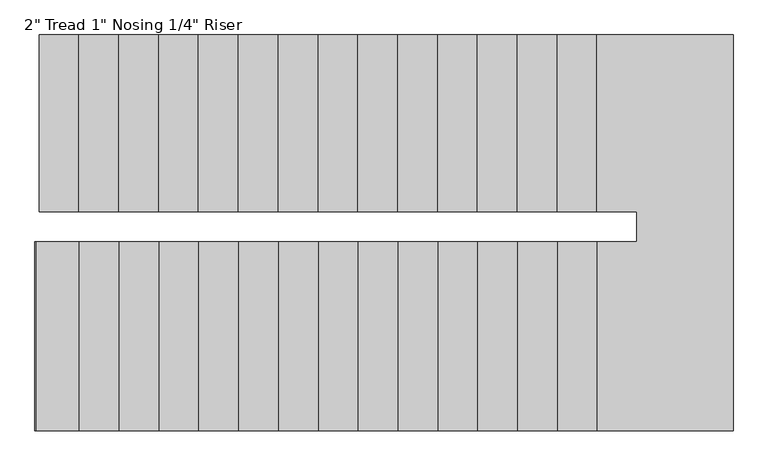
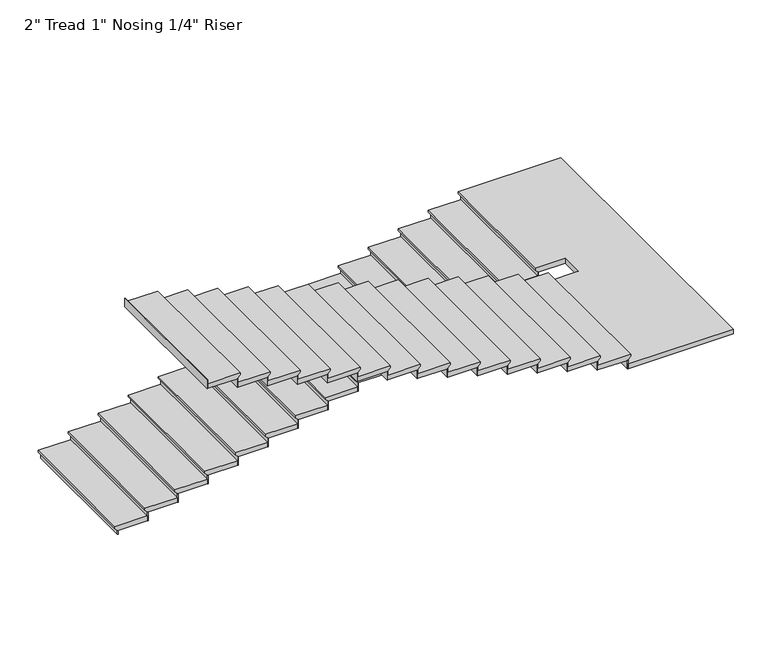
"""IFC4 building model written with IfcOpenShell, lengths in millimetres: stair flight geometry."""

from ifc_helpers import new_model, si_unit, origin, place, context, project, spatial, faceted_brep, source, transform, mapped, element, save


def stair_flight_8f1750f9(model_context):
    return source(origin(), model_context, "Body", "Brep", [
        faceted_brep([(-5254.0891351, 11154.2082924, 18360.39), (-5254.0891351, 11154.2082924, 18379.44), (-5254.0891351, 12506.0715905, 18379.44), (-5254.0891351, 12506.0715905, 18360.39), (-5228.6891351, 11154.2082924, 18334.99), (-5228.6891351, 12506.0715905, 18334.99), (-4923.8891351, 11154.2082924, 18379.44), (-4923.8891351, 12506.0715905, 18379.44), (-5228.6891351, 12506.0715905, 18328.64), (-4923.8891351, 12506.0715905, 18328.64), (-4923.8891351, 11154.2082924, 18328.64), (-5228.6891351, 11154.2082924, 18328.64)], [[[0, 1, 2, 3]], [[4, 0, 3, 5]], [[2, 1, 6, 7]], [[8, 9, 10, 11]], [[2, 7, 9, 8, 5, 3]], [[8, 11, 4, 5]], [[6, 1, 0, 4, 11, 10]], [[7, 6, 10, 9]]]),
        faceted_brep([(-5228.6891351, 11154.2082924, 18328.64), (-5228.6891351, 11154.2082924, 18288.0), (-5222.3391351, 11154.2082924, 18288.0), (-5222.3391351, 11154.2082924, 18328.64), (-5228.6891351, 12506.0715905, 18328.64), (-5222.3391351, 12506.0715905, 18328.64), (-5222.3391351, 12506.0715905, 18288.0), (-5228.6891351, 12506.0715905, 18288.0)], [[[0, 1, 2, 3]], [[4, 5, 6, 7]], [[1, 0, 4, 7]], [[2, 1, 7, 6]], [[3, 2, 6, 5]], [[0, 3, 5, 4]]]),
        faceted_brep([(-4923.8891351, 11154.2082924, 18420.08), (-4923.8891351, 11154.2082924, 18328.64), (-4917.5391351, 11154.2082924, 18328.64), (-4917.5391351, 11154.2082924, 18420.08), (-4923.8891351, 12506.0715905, 18420.08), (-4917.5391351, 12506.0715905, 18420.08), (-4917.5391351, 12506.0715905, 18328.64), (-4923.8891351, 12506.0715905, 18328.64)], [[[0, 1, 2, 3]], [[4, 5, 6, 7]], [[1, 0, 4, 7]], [[2, 1, 7, 6]], [[3, 2, 6, 5]], [[0, 3, 5, 4]]]),
        faceted_brep([(-4949.2891351, 12506.0715905, 18470.88), (-4949.2891351, 11154.2082924, 18470.88), (-4619.0891351, 11154.2082924, 18470.88), (-4619.0891351, 12506.0715905, 18470.88), (-4923.8891351, 12506.0715905, 18420.08), (-4619.0891351, 12506.0715905, 18420.08), (-4619.0891351, 11154.2082924, 18420.08), (-4923.8891351, 11154.2082924, 18420.08), (-4923.8891351, 12506.0715905, 18426.43), (-4949.2891351, 12506.0715905, 18451.83), (-4923.8891351, 11154.2082924, 18426.43), (-4949.2891351, 11154.2082924, 18451.83)], [[[0, 1, 2, 3]], [[4, 5, 6, 7]], [[0, 3, 5, 4, 8, 9]], [[4, 7, 10, 8]], [[2, 1, 11, 10, 7, 6]], [[3, 2, 6, 5]], [[11, 1, 0, 9]], [[10, 11, 9, 8]]]),
        faceted_brep([(-4619.0891351, 11154.2082924, 18511.52), (-4619.0891351, 11154.2082924, 18420.08), (-4612.7391351, 11154.2082924, 18420.08), (-4612.7391351, 11154.2082924, 18511.52), (-4619.0891351, 12506.0715905, 18511.52), (-4612.7391351, 12506.0715905, 18511.52), (-4612.7391351, 12506.0715905, 18420.08), (-4619.0891351, 12506.0715905, 18420.08)], [[[0, 1, 2, 3]], [[4, 5, 6, 7]], [[1, 0, 4, 7]], [[2, 1, 7, 6]], [[3, 2, 6, 5]], [[0, 3, 5, 4]]]),
        faceted_brep([(-4644.4891351, 12506.0715905, 18562.32), (-4644.4891351, 11154.2082924, 18562.32), (-4314.2891351, 11154.2082924, 18562.32), (-4314.2891351, 12506.0715905, 18562.32), (-4619.0891351, 12506.0715905, 18511.52), (-4314.2891351, 12506.0715905, 18511.52), (-4314.2891351, 11154.2082924, 18511.52), (-4619.0891351, 11154.2082924, 18511.52), (-4619.0891351, 12506.0715905, 18517.87), (-4644.4891351, 12506.0715905, 18543.27), (-4619.0891351, 11154.2082924, 18517.87), (-4644.4891351, 11154.2082924, 18543.27)], [[[0, 1, 2, 3]], [[4, 5, 6, 7]], [[0, 3, 5, 4, 8, 9]], [[4, 7, 10, 8]], [[2, 1, 11, 10, 7, 6]], [[3, 2, 6, 5]], [[11, 1, 0, 9]], [[10, 11, 9, 8]]]),
        faceted_brep([(-4314.2891351, 11154.2082924, 18602.96), (-4314.2891351, 11154.2082924, 18511.52), (-4307.9391351, 11154.2082924, 18511.52), (-4307.9391351, 11154.2082924, 18602.96), (-4314.2891351, 12506.0715905, 18602.96), (-4307.9391351, 12506.0715905, 18602.96), (-4307.9391351, 12506.0715905, 18511.52), (-4314.2891351, 12506.0715905, 18511.52)], [[[0, 1, 2, 3]], [[4, 5, 6, 7]], [[1, 0, 4, 7]], [[2, 1, 7, 6]], [[3, 2, 6, 5]], [[0, 3, 5, 4]]]),
        faceted_brep([(-4339.6891351, 12506.0715905, 18653.76), (-4339.6891351, 11154.2082924, 18653.76), (-4009.4891351, 11154.2082924, 18653.76), (-4009.4891351, 12506.0715905, 18653.76), (-4314.2891351, 12506.0715905, 18602.96), (-4009.4891351, 12506.0715905, 18602.96), (-4009.4891351, 11154.2082924, 18602.96), (-4314.2891351, 11154.2082924, 18602.96), (-4314.2891351, 12506.0715905, 18609.31), (-4339.6891351, 12506.0715905, 18634.71), (-4314.2891351, 11154.2082924, 18609.31), (-4339.6891351, 11154.2082924, 18634.71)], [[[0, 1, 2, 3]], [[4, 5, 6, 7]], [[0, 3, 5, 4, 8, 9]], [[4, 7, 10, 8]], [[2, 1, 11, 10, 7, 6]], [[3, 2, 6, 5]], [[11, 1, 0, 9]], [[10, 11, 9, 8]]]),
        faceted_brep([(-4009.4891351, 11154.2082924, 18694.4), (-4009.4891351, 11154.2082924, 18602.96), (-4003.1391351, 11154.2082924, 18602.96), (-4003.1391351, 11154.2082924, 18694.4), (-4009.4891351, 12506.0715905, 18694.4), (-4003.1391351, 12506.0715905, 18694.4), (-4003.1391351, 12506.0715905, 18602.96), (-4009.4891351, 12506.0715905, 18602.96)], [[[0, 1, 2, 3]], [[4, 5, 6, 7]], [[1, 0, 4, 7]], [[2, 1, 7, 6]], [[3, 2, 6, 5]], [[0, 3, 5, 4]]]),
        faceted_brep([(-4034.8891351, 12506.0715905, 18745.2), (-4034.8891351, 11154.2082924, 18745.2), (-3704.6891351, 11154.2082924, 18745.2), (-3704.6891351, 12506.0715905, 18745.2), (-4009.4891351, 12506.0715905, 18694.4), (-3704.6891351, 12506.0715905, 18694.4), (-3704.6891351, 11154.2082924, 18694.4), (-4009.4891351, 11154.2082924, 18694.4), (-4009.4891351, 12506.0715905, 18700.75), (-4034.8891351, 12506.0715905, 18726.15), (-4009.4891351, 11154.2082924, 18700.75), (-4034.8891351, 11154.2082924, 18726.15)], [[[0, 1, 2, 3]], [[4, 5, 6, 7]], [[0, 3, 5, 4, 8, 9]], [[4, 7, 10, 8]], [[2, 1, 11, 10, 7, 6]], [[3, 2, 6, 5]], [[11, 1, 0, 9]], [[10, 11, 9, 8]]]),
        faceted_brep([(-3704.6891351, 11154.2082924, 18785.84), (-3704.6891351, 11154.2082924, 18694.4), (-3698.3391351, 11154.2082924, 18694.4), (-3698.3391351, 11154.2082924, 18785.84), (-3704.6891351, 12506.0715905, 18785.84), (-3698.3391351, 12506.0715905, 18785.84), (-3698.3391351, 12506.0715905, 18694.4), (-3704.6891351, 12506.0715905, 18694.4)], [[[0, 1, 2, 3]], [[4, 5, 6, 7]], [[1, 0, 4, 7]], [[2, 1, 7, 6]], [[3, 2, 6, 5]], [[0, 3, 5, 4]]]),
        faceted_brep([(-3730.0891351, 12506.0715905, 18836.64), (-3730.0891351, 11154.2082924, 18836.64), (-3399.8891351, 11154.2082924, 18836.64), (-3399.8891351, 12506.0715905, 18836.64), (-3704.6891351, 12506.0715905, 18785.84), (-3399.8891351, 12506.0715905, 18785.84), (-3399.8891351, 11154.2082924, 18785.84), (-3704.6891351, 11154.2082924, 18785.84), (-3704.6891351, 12506.0715905, 18792.19), (-3730.0891351, 12506.0715905, 18817.59), (-3704.6891351, 11154.2082924, 18792.19), (-3730.0891351, 11154.2082924, 18817.59)], [[[0, 1, 2, 3]], [[4, 5, 6, 7]], [[0, 3, 5, 4, 8, 9]], [[4, 7, 10, 8]], [[2, 1, 11, 10, 7, 6]], [[3, 2, 6, 5]], [[11, 1, 0, 9]], [[10, 11, 9, 8]]]),
        faceted_brep([(-3399.8891351, 11154.2082924, 18877.28), (-3399.8891351, 11154.2082924, 18785.84), (-3393.5391351, 11154.2082924, 18785.84), (-3393.5391351, 11154.2082924, 18877.28), (-3399.8891351, 12506.0715905, 18877.28), (-3393.5391351, 12506.0715905, 18877.28), (-3393.5391351, 12506.0715905, 18785.84), (-3399.8891351, 12506.0715905, 18785.84)], [[[0, 1, 2, 3]], [[4, 5, 6, 7]], [[1, 0, 4, 7]], [[2, 1, 7, 6]], [[3, 2, 6, 5]], [[0, 3, 5, 4]]]),
        faceted_brep([(-3425.2891351, 12506.0715905, 18928.08), (-3425.2891351, 11154.2082924, 18928.08), (-3095.0891351, 11154.2082924, 18928.08), (-3095.0891351, 12506.0715905, 18928.08), (-3399.8891351, 12506.0715905, 18877.28), (-3095.0891351, 12506.0715905, 18877.28), (-3095.0891351, 11154.2082924, 18877.28), (-3399.8891351, 11154.2082924, 18877.28), (-3399.8891351, 12506.0715905, 18883.63), (-3425.2891351, 12506.0715905, 18909.03), (-3399.8891351, 11154.2082924, 18883.63), (-3425.2891351, 11154.2082924, 18909.03)], [[[0, 1, 2, 3]], [[4, 5, 6, 7]], [[0, 3, 5, 4, 8, 9]], [[4, 7, 10, 8]], [[2, 1, 11, 10, 7, 6]], [[3, 2, 6, 5]], [[11, 1, 0, 9]], [[10, 11, 9, 8]]]),
        faceted_brep([(-3095.0891351, 11154.2082924, 18968.72), (-3095.0891351, 11154.2082924, 18877.28), (-3088.7391351, 11154.2082924, 18877.28), (-3088.7391351, 11154.2082924, 18968.72), (-3095.0891351, 12506.0715905, 18968.72), (-3088.7391351, 12506.0715905, 18968.72), (-3088.7391351, 12506.0715905, 18877.28), (-3095.0891351, 12506.0715905, 18877.28)], [[[0, 1, 2, 3]], [[4, 5, 6, 7]], [[1, 0, 4, 7]], [[2, 1, 7, 6]], [[3, 2, 6, 5]], [[0, 3, 5, 4]]]),
        faceted_brep([(-3120.4891351, 12506.0715905, 19019.52), (-3120.4891351, 11154.2082924, 19019.52), (-2790.2891351, 11154.2082924, 19019.52), (-2790.2891351, 12506.0715905, 19019.52), (-3095.0891351, 12506.0715905, 18968.72), (-2790.2891351, 12506.0715905, 18968.72), (-2790.2891351, 11154.2082924, 18968.72), (-3095.0891351, 11154.2082924, 18968.72), (-3095.0891351, 12506.0715905, 18975.07), (-3120.4891351, 12506.0715905, 19000.47), (-3095.0891351, 11154.2082924, 18975.07), (-3120.4891351, 11154.2082924, 19000.47)], [[[0, 1, 2, 3]], [[4, 5, 6, 7]], [[0, 3, 5, 4, 8, 9]], [[4, 7, 10, 8]], [[2, 1, 11, 10, 7, 6]], [[3, 2, 6, 5]], [[11, 1, 0, 9]], [[10, 11, 9, 8]]]),
        faceted_brep([(-2790.2891351, 11154.2082924, 19060.16), (-2790.2891351, 11154.2082924, 18968.72), (-2783.9391351, 11154.2082924, 18968.72), (-2783.9391351, 11154.2082924, 19060.16), (-2790.2891351, 12506.0715905, 19060.16), (-2783.9391351, 12506.0715905, 19060.16), (-2783.9391351, 12506.0715905, 18968.72), (-2790.2891351, 12506.0715905, 18968.72)], [[[0, 1, 2, 3]], [[4, 5, 6, 7]], [[1, 0, 4, 7]], [[2, 1, 7, 6]], [[3, 2, 6, 5]], [[0, 3, 5, 4]]]),
        faceted_brep([(-2815.6891351, 12506.0715905, 19110.96), (-2815.6891351, 11154.2082924, 19110.96), (-2485.4891351, 11154.2082924, 19110.96), (-2485.4891351, 12506.0715905, 19110.96), (-2790.2891351, 12506.0715905, 19060.16), (-2485.4891351, 12506.0715905, 19060.16), (-2485.4891351, 11154.2082924, 19060.16), (-2790.2891351, 11154.2082924, 19060.16), (-2790.2891351, 12506.0715905, 19066.51), (-2815.6891351, 12506.0715905, 19091.91), (-2790.2891351, 11154.2082924, 19066.51), (-2815.6891351, 11154.2082924, 19091.91)], [[[0, 1, 2, 3]], [[4, 5, 6, 7]], [[0, 3, 5, 4, 8, 9]], [[4, 7, 10, 8]], [[2, 1, 11, 10, 7, 6]], [[3, 2, 6, 5]], [[11, 1, 0, 9]], [[10, 11, 9, 8]]]),
        faceted_brep([(-2485.4891351, 11154.2082924, 19151.6), (-2485.4891351, 11154.2082924, 19060.16), (-2479.1391351, 11154.2082924, 19060.16), (-2479.1391351, 11154.2082924, 19151.6), (-2485.4891351, 12506.0715905, 19151.6), (-2479.1391351, 12506.0715905, 19151.6), (-2479.1391351, 12506.0715905, 19060.16), (-2485.4891351, 12506.0715905, 19060.16)], [[[0, 1, 2, 3]], [[4, 5, 6, 7]], [[1, 0, 4, 7]], [[2, 1, 7, 6]], [[3, 2, 6, 5]], [[0, 3, 5, 4]]]),
        faceted_brep([(-2510.8891351, 12506.0715905, 19202.4), (-2510.8891351, 11154.2082924, 19202.4), (-2180.6891351, 11154.2082924, 19202.4), (-2180.6891351, 12506.0715905, 19202.4), (-2485.4891351, 12506.0715905, 19151.6), (-2180.6891351, 12506.0715905, 19151.6), (-2180.6891351, 11154.2082924, 19151.6), (-2485.4891351, 11154.2082924, 19151.6), (-2485.4891351, 12506.0715905, 19157.95), (-2510.8891351, 12506.0715905, 19183.35), (-2485.4891351, 11154.2082924, 19157.95), (-2510.8891351, 11154.2082924, 19183.35)], [[[0, 1, 2, 3]], [[4, 5, 6, 7]], [[0, 3, 5, 4, 8, 9]], [[4, 7, 10, 8]], [[2, 1, 11, 10, 7, 6]], [[3, 2, 6, 5]], [[11, 1, 0, 9]], [[10, 11, 9, 8]]]),
        faceted_brep([(-2180.6891351, 11154.2082924, 19243.04), (-2180.6891351, 11154.2082924, 19151.6), (-2174.3391351, 11154.2082924, 19151.6), (-2174.3391351, 11154.2082924, 19243.04), (-2180.6891351, 12506.0715905, 19243.04), (-2174.3391351, 12506.0715905, 19243.04), (-2174.3391351, 12506.0715905, 19151.6), (-2180.6891351, 12506.0715905, 19151.6)], [[[0, 1, 2, 3]], [[4, 5, 6, 7]], [[1, 0, 4, 7]], [[2, 1, 7, 6]], [[3, 2, 6, 5]], [[0, 3, 5, 4]]]),
        faceted_brep([(-2206.0891351, 12506.0715905, 19293.84), (-2206.0891351, 11154.2082924, 19293.84), (-1875.8891351, 11154.2082924, 19293.84), (-1875.8891351, 12506.0715905, 19293.84), (-2180.6891351, 12506.0715905, 19243.04), (-1875.8891351, 12506.0715905, 19243.04), (-1875.8891351, 11154.2082924, 19243.04), (-2180.6891351, 11154.2082924, 19243.04), (-2180.6891351, 12506.0715905, 19249.39), (-2206.0891351, 12506.0715905, 19274.79), (-2180.6891351, 11154.2082924, 19249.39), (-2206.0891351, 11154.2082924, 19274.79)], [[[0, 1, 2, 3]], [[4, 5, 6, 7]], [[0, 3, 5, 4, 8, 9]], [[4, 7, 10, 8]], [[2, 1, 11, 10, 7, 6]], [[3, 2, 6, 5]], [[11, 1, 0, 9]], [[10, 11, 9, 8]]]),
        faceted_brep([(-1875.8891351, 11154.2082924, 19334.48), (-1875.8891351, 11154.2082924, 19243.04), (-1869.5391351, 11154.2082924, 19243.04), (-1869.5391351, 11154.2082924, 19334.48), (-1875.8891351, 12506.0715905, 19334.48), (-1869.5391351, 12506.0715905, 19334.48), (-1869.5391351, 12506.0715905, 19243.04), (-1875.8891351, 12506.0715905, 19243.04)], [[[0, 1, 2, 3]], [[4, 5, 6, 7]], [[1, 0, 4, 7]], [[2, 1, 7, 6]], [[3, 2, 6, 5]], [[0, 3, 5, 4]]]),
        faceted_brep([(-1901.2891351, 12506.0715905, 19385.28), (-1901.2891351, 11154.2082924, 19385.28), (-1571.0891351, 11154.2082924, 19385.28), (-1571.0891351, 12506.0715905, 19385.28), (-1875.8891351, 12506.0715905, 19334.48), (-1571.0891351, 12506.0715905, 19334.48), (-1571.0891351, 11154.2082924, 19334.48), (-1875.8891351, 11154.2082924, 19334.48), (-1875.8891351, 12506.0715905, 19340.83), (-1901.2891351, 12506.0715905, 19366.23), (-1875.8891351, 11154.2082924, 19340.83), (-1901.2891351, 11154.2082924, 19366.23)], [[[0, 1, 2, 3]], [[4, 5, 6, 7]], [[0, 3, 5, 4, 8, 9]], [[4, 7, 10, 8]], [[2, 1, 11, 10, 7, 6]], [[3, 2, 6, 5]], [[11, 1, 0, 9]], [[10, 11, 9, 8]]]),
        faceted_brep([(-1571.0891351, 11154.2082924, 19425.92), (-1571.0891351, 11154.2082924, 19334.48), (-1564.7391351, 11154.2082924, 19334.48), (-1564.7391351, 11154.2082924, 19425.92), (-1571.0891351, 12506.0715905, 19425.92), (-1564.7391351, 12506.0715905, 19425.92), (-1564.7391351, 12506.0715905, 19334.48), (-1571.0891351, 12506.0715905, 19334.48)], [[[0, 1, 2, 3]], [[4, 5, 6, 7]], [[1, 0, 4, 7]], [[2, 1, 7, 6]], [[3, 2, 6, 5]], [[0, 3, 5, 4]]]),
        faceted_brep([(-1596.4891351, 12506.0715905, 19476.72), (-1596.4891351, 11154.2082924, 19476.72), (-1266.2891351, 11154.2082924, 19476.72), (-1266.2891351, 12506.0715905, 19476.72), (-1571.0891351, 12506.0715905, 19425.92), (-1266.2891351, 12506.0715905, 19425.92), (-1266.2891351, 11154.2082924, 19425.92), (-1571.0891351, 11154.2082924, 19425.92), (-1571.0891351, 12506.0715905, 19432.27), (-1596.4891351, 12506.0715905, 19457.67), (-1571.0891351, 11154.2082924, 19432.27), (-1596.4891351, 11154.2082924, 19457.67)], [[[0, 1, 2, 3]], [[4, 5, 6, 7]], [[0, 3, 5, 4, 8, 9]], [[4, 7, 10, 8]], [[2, 1, 11, 10, 7, 6]], [[3, 2, 6, 5]], [[11, 1, 0, 9]], [[10, 11, 9, 8]]]),
        faceted_brep([(-1266.2891351, 11154.2082924, 19517.36), (-1266.2891351, 11154.2082924, 19425.92), (-1259.9391351, 11154.2082924, 19425.92), (-1259.9391351, 11154.2082924, 19517.36), (-1266.2891351, 12506.0715905, 19517.36), (-1259.9391351, 12506.0715905, 19517.36), (-1259.9391351, 12506.0715905, 19425.92), (-1266.2891351, 12506.0715905, 19425.92)], [[[0, 1, 2, 3]], [[4, 5, 6, 7]], [[1, 0, 4, 7]], [[2, 1, 7, 6]], [[3, 2, 6, 5]], [[0, 3, 5, 4]]]),
        faceted_brep([(-1291.6891351, 12506.0715905, 19568.16), (-1291.6891351, 11154.2082924, 19568.16), (-961.4891351, 11154.2082924, 19568.16), (-961.4891351, 12506.0715905, 19568.16), (-1266.2891351, 12506.0715905, 19517.36), (-961.4891351, 12506.0715905, 19517.36), (-961.4891351, 11154.2082924, 19517.36), (-1266.2891351, 11154.2082924, 19517.36), (-1266.2891351, 12506.0715905, 19523.71), (-1291.6891351, 12506.0715905, 19549.11), (-1266.2891351, 11154.2082924, 19523.71), (-1291.6891351, 11154.2082924, 19549.11)], [[[0, 1, 2, 3]], [[4, 5, 6, 7]], [[0, 3, 5, 4, 8, 9]], [[4, 7, 10, 8]], [[2, 1, 11, 10, 7, 6]], [[3, 2, 6, 5]], [[11, 1, 0, 9]], [[10, 11, 9, 8]]]),
        faceted_brep([(-961.4891351, 11154.2082924, 19608.8), (-961.4891351, 11154.2082924, 19517.36), (-955.1391351, 11154.2082924, 19517.36), (-955.1391351, 11154.2082924, 19608.8), (-961.4891351, 12506.0715905, 19608.8), (-955.1391351, 12506.0715905, 19608.8), (-955.1391351, 12506.0715905, 19517.36), (-961.4891351, 12506.0715905, 19517.36)], [[[0, 1, 2, 3]], [[4, 5, 6, 7]], [[1, 0, 4, 7]], [[2, 1, 7, 6]], [[3, 2, 6, 5]], [[0, 3, 5, 4]]]),
        faceted_brep([(-1012.2891351, 9478.4949943, 19659.6), (54.5108649, 9478.4949943, 19659.6), (54.5108649, 12506.0715905, 19659.6), (-986.8891351, 12506.0715905, 19659.6), (-986.8891351, 11154.2082924, 19659.6), (-682.0891351, 11154.2082924, 19659.6), (-682.0891351, 10925.6082924, 19659.6), (-1012.2891351, 10925.6082924, 19659.6), (54.5108649, 9478.4949943, 19608.8), (-1012.2891351, 9478.4949943, 19608.8), (-1012.2891351, 10925.6082924, 19608.8), (-682.0891351, 10925.6082924, 19608.8), (-682.0891351, 11154.2082924, 19608.8), (-961.4891351, 11154.2082924, 19608.8), (-961.4891351, 12506.0715905, 19608.8), (54.5108649, 12506.0715905, 19608.8), (-961.4891351, 12506.0715905, 19615.15), (-986.8891351, 12506.0715905, 19640.55), (-961.4891351, 11154.2082924, 19615.15), (-986.8891351, 11154.2082924, 19640.55)], [[[0, 1, 2, 3, 4, 5, 6, 7]], [[8, 9, 10, 11, 12, 13, 14, 15]], [[1, 0, 9, 8]], [[2, 1, 8, 15]], [[3, 2, 15, 14, 16, 17]], [[14, 13, 18, 16]], [[5, 4, 19, 18, 13, 12]], [[6, 5, 12, 11]], [[7, 6, 11, 10]], [[0, 7, 10, 9]], [[19, 4, 3, 17]], [[18, 19, 17, 16]]]),
        faceted_brep([(-1012.2891351, 10925.6082924, 19700.24), (-1012.2891351, 10925.6082924, 19608.8), (-1018.6391351, 10925.6082924, 19608.8), (-1018.6391351, 10925.6082924, 19700.24), (-1012.2891351, 9478.4949943, 19700.24), (-1018.6391351, 9478.4949943, 19700.24), (-1018.6391351, 9478.4949943, 19608.8), (-1012.2891351, 9478.4949943, 19608.8)], [[[0, 1, 2, 3]], [[4, 5, 6, 7]], [[1, 0, 4, 7]], [[2, 1, 7, 6]], [[3, 2, 6, 5]], [[0, 3, 5, 4]]]),
        faceted_brep([(-986.8891351, 9478.4949943, 19751.04), (-986.8891351, 10925.6082924, 19751.04), (-1317.0891351, 10925.6082924, 19751.04), (-1317.0891351, 9478.4949943, 19751.04), (-1012.2891351, 9478.4949943, 19700.24), (-1317.0891351, 9478.4949943, 19700.24), (-1317.0891351, 10925.6082924, 19700.24), (-1012.2891351, 10925.6082924, 19700.24), (-1012.2891351, 9478.4949943, 19706.59), (-986.8891351, 9478.4949943, 19731.99), (-1012.2891351, 10925.6082924, 19706.59), (-986.8891351, 10925.6082924, 19731.99)], [[[0, 1, 2, 3]], [[4, 5, 6, 7]], [[0, 3, 5, 4, 8, 9]], [[4, 7, 10, 8]], [[2, 1, 11, 10, 7, 6]], [[3, 2, 6, 5]], [[11, 1, 0, 9]], [[10, 11, 9, 8]]]),
        faceted_brep([(-1317.0891351, 10925.6082924, 19791.68), (-1317.0891351, 10925.6082924, 19700.24), (-1323.4391351, 10925.6082924, 19700.24), (-1323.4391351, 10925.6082924, 19791.68), (-1317.0891351, 9478.4949943, 19791.68), (-1323.4391351, 9478.4949943, 19791.68), (-1323.4391351, 9478.4949943, 19700.24), (-1317.0891351, 9478.4949943, 19700.24)], [[[0, 1, 2, 3]], [[4, 5, 6, 7]], [[1, 0, 4, 7]], [[2, 1, 7, 6]], [[3, 2, 6, 5]], [[0, 3, 5, 4]]]),
        faceted_brep([(-1291.6891351, 9478.4949943, 19842.48), (-1291.6891351, 10925.6082924, 19842.48), (-1621.8891351, 10925.6082924, 19842.48), (-1621.8891351, 9478.4949943, 19842.48), (-1317.0891351, 9478.4949943, 19791.68), (-1621.8891351, 9478.4949943, 19791.68), (-1621.8891351, 10925.6082924, 19791.68), (-1317.0891351, 10925.6082924, 19791.68), (-1317.0891351, 9478.4949943, 19798.03), (-1291.6891351, 9478.4949943, 19823.43), (-1317.0891351, 10925.6082924, 19798.03), (-1291.6891351, 10925.6082924, 19823.43)], [[[0, 1, 2, 3]], [[4, 5, 6, 7]], [[0, 3, 5, 4, 8, 9]], [[4, 7, 10, 8]], [[2, 1, 11, 10, 7, 6]], [[3, 2, 6, 5]], [[11, 1, 0, 9]], [[10, 11, 9, 8]]]),
        faceted_brep([(-1621.8891351, 10925.6082924, 19883.12), (-1621.8891351, 10925.6082924, 19791.68), (-1628.2391351, 10925.6082924, 19791.68), (-1628.2391351, 10925.6082924, 19883.12), (-1621.8891351, 9478.4949943, 19883.12), (-1628.2391351, 9478.4949943, 19883.12), (-1628.2391351, 9478.4949943, 19791.68), (-1621.8891351, 9478.4949943, 19791.68)], [[[0, 1, 2, 3]], [[4, 5, 6, 7]], [[1, 0, 4, 7]], [[2, 1, 7, 6]], [[3, 2, 6, 5]], [[0, 3, 5, 4]]]),
        faceted_brep([(-1596.4891351, 9478.4949943, 19933.92), (-1596.4891351, 10925.6082924, 19933.92), (-1926.6891351, 10925.6082924, 19933.92), (-1926.6891351, 9478.4949943, 19933.92), (-1621.8891351, 9478.4949943, 19883.12), (-1926.6891351, 9478.4949943, 19883.12), (-1926.6891351, 10925.6082924, 19883.12), (-1621.8891351, 10925.6082924, 19883.12), (-1621.8891351, 9478.4949943, 19889.47), (-1596.4891351, 9478.4949943, 19914.87), (-1621.8891351, 10925.6082924, 19889.47), (-1596.4891351, 10925.6082924, 19914.87)], [[[0, 1, 2, 3]], [[4, 5, 6, 7]], [[0, 3, 5, 4, 8, 9]], [[4, 7, 10, 8]], [[2, 1, 11, 10, 7, 6]], [[3, 2, 6, 5]], [[11, 1, 0, 9]], [[10, 11, 9, 8]]]),
        faceted_brep([(-1926.6891351, 10925.6082924, 19974.56), (-1926.6891351, 10925.6082924, 19883.12), (-1933.0391351, 10925.6082924, 19883.12), (-1933.0391351, 10925.6082924, 19974.56), (-1926.6891351, 9478.4949943, 19974.56), (-1933.0391351, 9478.4949943, 19974.56), (-1933.0391351, 9478.4949943, 19883.12), (-1926.6891351, 9478.4949943, 19883.12)], [[[0, 1, 2, 3]], [[4, 5, 6, 7]], [[1, 0, 4, 7]], [[2, 1, 7, 6]], [[3, 2, 6, 5]], [[0, 3, 5, 4]]]),
        faceted_brep([(-1901.2891351, 9478.4949943, 20025.36), (-1901.2891351, 10925.6082924, 20025.36), (-2231.4891351, 10925.6082924, 20025.36), (-2231.4891351, 9478.4949943, 20025.36), (-1926.6891351, 9478.4949943, 19974.56), (-2231.4891351, 9478.4949943, 19974.56), (-2231.4891351, 10925.6082924, 19974.56), (-1926.6891351, 10925.6082924, 19974.56), (-1926.6891351, 9478.4949943, 19980.91), (-1901.2891351, 9478.4949943, 20006.31), (-1926.6891351, 10925.6082924, 19980.91), (-1901.2891351, 10925.6082924, 20006.31)], [[[0, 1, 2, 3]], [[4, 5, 6, 7]], [[0, 3, 5, 4, 8, 9]], [[4, 7, 10, 8]], [[2, 1, 11, 10, 7, 6]], [[3, 2, 6, 5]], [[11, 1, 0, 9]], [[10, 11, 9, 8]]]),
        faceted_brep([(-2231.4891351, 10925.6082924, 20066.0), (-2231.4891351, 10925.6082924, 19974.56), (-2237.8391351, 10925.6082924, 19974.56), (-2237.8391351, 10925.6082924, 20066.0), (-2231.4891351, 9478.4949943, 20066.0), (-2237.8391351, 9478.4949943, 20066.0), (-2237.8391351, 9478.4949943, 19974.56), (-2231.4891351, 9478.4949943, 19974.56)], [[[0, 1, 2, 3]], [[4, 5, 6, 7]], [[1, 0, 4, 7]], [[2, 1, 7, 6]], [[3, 2, 6, 5]], [[0, 3, 5, 4]]]),
        faceted_brep([(-2206.0891351, 9478.4949943, 20116.8), (-2206.0891351, 10925.6082924, 20116.8), (-2536.2891351, 10925.6082924, 20116.8), (-2536.2891351, 9478.4949943, 20116.8), (-2231.4891351, 9478.4949943, 20066.0), (-2536.2891351, 9478.4949943, 20066.0), (-2536.2891351, 10925.6082924, 20066.0), (-2231.4891351, 10925.6082924, 20066.0), (-2231.4891351, 9478.4949943, 20072.35), (-2206.0891351, 9478.4949943, 20097.75), (-2231.4891351, 10925.6082924, 20072.35), (-2206.0891351, 10925.6082924, 20097.75)], [[[0, 1, 2, 3]], [[4, 5, 6, 7]], [[0, 3, 5, 4, 8, 9]], [[4, 7, 10, 8]], [[2, 1, 11, 10, 7, 6]], [[3, 2, 6, 5]], [[11, 1, 0, 9]], [[10, 11, 9, 8]]]),
        faceted_brep([(-2536.2891351, 10925.6082924, 20157.44), (-2536.2891351, 10925.6082924, 20066.0), (-2542.6391351, 10925.6082924, 20066.0), (-2542.6391351, 10925.6082924, 20157.44), (-2536.2891351, 9478.4949943, 20157.44), (-2542.6391351, 9478.4949943, 20157.44), (-2542.6391351, 9478.4949943, 20066.0), (-2536.2891351, 9478.4949943, 20066.0)], [[[0, 1, 2, 3]], [[4, 5, 6, 7]], [[1, 0, 4, 7]], [[2, 1, 7, 6]], [[3, 2, 6, 5]], [[0, 3, 5, 4]]]),
        faceted_brep([(-2510.8891351, 9478.4949943, 20208.24), (-2510.8891351, 10925.6082924, 20208.24), (-2841.0891351, 10925.6082924, 20208.24), (-2841.0891351, 9478.4949943, 20208.24), (-2536.2891351, 9478.4949943, 20157.44), (-2841.0891351, 9478.4949943, 20157.44), (-2841.0891351, 10925.6082924, 20157.44), (-2536.2891351, 10925.6082924, 20157.44), (-2536.2891351, 9478.4949943, 20163.79), (-2510.8891351, 9478.4949943, 20189.19), (-2536.2891351, 10925.6082924, 20163.79), (-2510.8891351, 10925.6082924, 20189.19)], [[[0, 1, 2, 3]], [[4, 5, 6, 7]], [[0, 3, 5, 4, 8, 9]], [[4, 7, 10, 8]], [[2, 1, 11, 10, 7, 6]], [[3, 2, 6, 5]], [[11, 1, 0, 9]], [[10, 11, 9, 8]]]),
        faceted_brep([(-2841.0891351, 10925.6082924, 20248.88), (-2841.0891351, 10925.6082924, 20157.44), (-2847.4391351, 10925.6082924, 20157.44), (-2847.4391351, 10925.6082924, 20248.88), (-2841.0891351, 9478.4949943, 20248.88), (-2847.4391351, 9478.4949943, 20248.88), (-2847.4391351, 9478.4949943, 20157.44), (-2841.0891351, 9478.4949943, 20157.44)], [[[0, 1, 2, 3]], [[4, 5, 6, 7]], [[1, 0, 4, 7]], [[2, 1, 7, 6]], [[3, 2, 6, 5]], [[0, 3, 5, 4]]]),
        faceted_brep([(-2815.6891351, 9478.4949943, 20299.68), (-2815.6891351, 10925.6082924, 20299.68), (-3145.8891351, 10925.6082924, 20299.68), (-3145.8891351, 9478.4949943, 20299.68), (-2841.0891351, 9478.4949943, 20248.88), (-3145.8891351, 9478.4949943, 20248.88), (-3145.8891351, 10925.6082924, 20248.88), (-2841.0891351, 10925.6082924, 20248.88), (-2841.0891351, 9478.4949943, 20255.23), (-2815.6891351, 9478.4949943, 20280.63), (-2841.0891351, 10925.6082924, 20255.23), (-2815.6891351, 10925.6082924, 20280.63)], [[[0, 1, 2, 3]], [[4, 5, 6, 7]], [[0, 3, 5, 4, 8, 9]], [[4, 7, 10, 8]], [[2, 1, 11, 10, 7, 6]], [[3, 2, 6, 5]], [[11, 1, 0, 9]], [[10, 11, 9, 8]]]),
        faceted_brep([(-3145.8891351, 10925.6082924, 20340.32), (-3145.8891351, 10925.6082924, 20248.88), (-3152.2391351, 10925.6082924, 20248.88), (-3152.2391351, 10925.6082924, 20340.32), (-3145.8891351, 9478.4949943, 20340.32), (-3152.2391351, 9478.4949943, 20340.32), (-3152.2391351, 9478.4949943, 20248.88), (-3145.8891351, 9478.4949943, 20248.88)], [[[0, 1, 2, 3]], [[4, 5, 6, 7]], [[1, 0, 4, 7]], [[2, 1, 7, 6]], [[3, 2, 6, 5]], [[0, 3, 5, 4]]]),
        faceted_brep([(-3120.4891351, 9478.4949943, 20391.12), (-3120.4891351, 10925.6082924, 20391.12), (-3450.6891351, 10925.6082924, 20391.12), (-3450.6891351, 9478.4949943, 20391.12), (-3145.8891351, 9478.4949943, 20340.32), (-3450.6891351, 9478.4949943, 20340.32), (-3450.6891351, 10925.6082924, 20340.32), (-3145.8891351, 10925.6082924, 20340.32), (-3145.8891351, 9478.4949943, 20346.67), (-3120.4891351, 9478.4949943, 20372.07), (-3145.8891351, 10925.6082924, 20346.67), (-3120.4891351, 10925.6082924, 20372.07)], [[[0, 1, 2, 3]], [[4, 5, 6, 7]], [[0, 3, 5, 4, 8, 9]], [[4, 7, 10, 8]], [[2, 1, 11, 10, 7, 6]], [[3, 2, 6, 5]], [[11, 1, 0, 9]], [[10, 11, 9, 8]]]),
        faceted_brep([(-3450.6891351, 10925.6082924, 20431.76), (-3450.6891351, 10925.6082924, 20340.32), (-3457.0391351, 10925.6082924, 20340.32), (-3457.0391351, 10925.6082924, 20431.76), (-3450.6891351, 9478.4949943, 20431.76), (-3457.0391351, 9478.4949943, 20431.76), (-3457.0391351, 9478.4949943, 20340.32), (-3450.6891351, 9478.4949943, 20340.32)], [[[0, 1, 2, 3]], [[4, 5, 6, 7]], [[1, 0, 4, 7]], [[2, 1, 7, 6]], [[3, 2, 6, 5]], [[0, 3, 5, 4]]]),
        faceted_brep([(-3425.2891351, 9478.4949943, 20482.56), (-3425.2891351, 10925.6082924, 20482.56), (-3755.4891351, 10925.6082924, 20482.56), (-3755.4891351, 9478.4949943, 20482.56), (-3450.6891351, 9478.4949943, 20431.76), (-3755.4891351, 9478.4949943, 20431.76), (-3755.4891351, 10925.6082924, 20431.76), (-3450.6891351, 10925.6082924, 20431.76), (-3450.6891351, 9478.4949943, 20438.11), (-3425.2891351, 9478.4949943, 20463.51), (-3450.6891351, 10925.6082924, 20438.11), (-3425.2891351, 10925.6082924, 20463.51)], [[[0, 1, 2, 3]], [[4, 5, 6, 7]], [[0, 3, 5, 4, 8, 9]], [[4, 7, 10, 8]], [[2, 1, 11, 10, 7, 6]], [[3, 2, 6, 5]], [[11, 1, 0, 9]], [[10, 11, 9, 8]]]),
        faceted_brep([(-3755.4891351, 10925.6082924, 20523.2), (-3755.4891351, 10925.6082924, 20431.76), (-3761.8391351, 10925.6082924, 20431.76), (-3761.8391351, 10925.6082924, 20523.2), (-3755.4891351, 9478.4949943, 20523.2), (-3761.8391351, 9478.4949943, 20523.2), (-3761.8391351, 9478.4949943, 20431.76), (-3755.4891351, 9478.4949943, 20431.76)], [[[0, 1, 2, 3]], [[4, 5, 6, 7]], [[1, 0, 4, 7]], [[2, 1, 7, 6]], [[3, 2, 6, 5]], [[0, 3, 5, 4]]]),
        faceted_brep([(-3730.0891351, 9478.4949943, 20574.0), (-3730.0891351, 10925.6082924, 20574.0), (-4060.2891351, 10925.6082924, 20574.0), (-4060.2891351, 9478.4949943, 20574.0), (-3755.4891351, 9478.4949943, 20523.2), (-4060.2891351, 9478.4949943, 20523.2), (-4060.2891351, 10925.6082924, 20523.2), (-3755.4891351, 10925.6082924, 20523.2), (-3755.4891351, 9478.4949943, 20529.55), (-3730.0891351, 9478.4949943, 20554.95), (-3755.4891351, 10925.6082924, 20529.55), (-3730.0891351, 10925.6082924, 20554.95)], [[[0, 1, 2, 3]], [[4, 5, 6, 7]], [[0, 3, 5, 4, 8, 9]], [[4, 7, 10, 8]], [[2, 1, 11, 10, 7, 6]], [[3, 2, 6, 5]], [[11, 1, 0, 9]], [[10, 11, 9, 8]]]),
        faceted_brep([(-4060.2891351, 10925.6082924, 20614.64), (-4060.2891351, 10925.6082924, 20523.2), (-4066.6391351, 10925.6082924, 20523.2), (-4066.6391351, 10925.6082924, 20614.64), (-4060.2891351, 9478.4949943, 20614.64), (-4066.6391351, 9478.4949943, 20614.64), (-4066.6391351, 9478.4949943, 20523.2), (-4060.2891351, 9478.4949943, 20523.2)], [[[0, 1, 2, 3]], [[4, 5, 6, 7]], [[1, 0, 4, 7]], [[2, 1, 7, 6]], [[3, 2, 6, 5]], [[0, 3, 5, 4]]]),
        faceted_brep([(-4034.8891351, 9478.4949943, 20665.44), (-4034.8891351, 10925.6082924, 20665.44), (-4365.0891351, 10925.6082924, 20665.44), (-4365.0891351, 9478.4949943, 20665.44), (-4060.2891351, 9478.4949943, 20614.64), (-4365.0891351, 9478.4949943, 20614.64), (-4365.0891351, 10925.6082924, 20614.64), (-4060.2891351, 10925.6082924, 20614.64), (-4060.2891351, 9478.4949943, 20620.99), (-4034.8891351, 9478.4949943, 20646.39), (-4060.2891351, 10925.6082924, 20620.99), (-4034.8891351, 10925.6082924, 20646.39)], [[[0, 1, 2, 3]], [[4, 5, 6, 7]], [[0, 3, 5, 4, 8, 9]], [[4, 7, 10, 8]], [[2, 1, 11, 10, 7, 6]], [[3, 2, 6, 5]], [[11, 1, 0, 9]], [[10, 11, 9, 8]]]),
        faceted_brep([(-4365.0891351, 10925.6082924, 20706.08), (-4365.0891351, 10925.6082924, 20614.64), (-4371.4391351, 10925.6082924, 20614.64), (-4371.4391351, 10925.6082924, 20706.08), (-4365.0891351, 9478.4949943, 20706.08), (-4371.4391351, 9478.4949943, 20706.08), (-4371.4391351, 9478.4949943, 20614.64), (-4365.0891351, 9478.4949943, 20614.64)], [[[0, 1, 2, 3]], [[4, 5, 6, 7]], [[1, 0, 4, 7]], [[2, 1, 7, 6]], [[3, 2, 6, 5]], [[0, 3, 5, 4]]]),
        faceted_brep([(-4339.6891351, 9478.4949943, 20756.88), (-4339.6891351, 10925.6082924, 20756.88), (-4669.8891351, 10925.6082924, 20756.88), (-4669.8891351, 9478.4949943, 20756.88), (-4365.0891351, 9478.4949943, 20706.08), (-4669.8891351, 9478.4949943, 20706.08), (-4669.8891351, 10925.6082924, 20706.08), (-4365.0891351, 10925.6082924, 20706.08), (-4365.0891351, 9478.4949943, 20712.43), (-4339.6891351, 9478.4949943, 20737.83), (-4365.0891351, 10925.6082924, 20712.43), (-4339.6891351, 10925.6082924, 20737.83)], [[[0, 1, 2, 3]], [[4, 5, 6, 7]], [[0, 3, 5, 4, 8, 9]], [[4, 7, 10, 8]], [[2, 1, 11, 10, 7, 6]], [[3, 2, 6, 5]], [[11, 1, 0, 9]], [[10, 11, 9, 8]]]),
        faceted_brep([(-4669.8891351, 10925.6082924, 20797.52), (-4669.8891351, 10925.6082924, 20706.08), (-4676.2391351, 10925.6082924, 20706.08), (-4676.2391351, 10925.6082924, 20797.52), (-4669.8891351, 9478.4949943, 20797.52), (-4676.2391351, 9478.4949943, 20797.52), (-4676.2391351, 9478.4949943, 20706.08), (-4669.8891351, 9478.4949943, 20706.08)], [[[0, 1, 2, 3]], [[4, 5, 6, 7]], [[1, 0, 4, 7]], [[2, 1, 7, 6]], [[3, 2, 6, 5]], [[0, 3, 5, 4]]]),
        faceted_brep([(-4644.4891351, 9478.4949943, 20848.32), (-4644.4891351, 10925.6082924, 20848.32), (-4974.6891351, 10925.6082924, 20848.32), (-4974.6891351, 9478.4949943, 20848.32), (-4669.8891351, 9478.4949943, 20797.52), (-4974.6891351, 9478.4949943, 20797.52), (-4974.6891351, 10925.6082924, 20797.52), (-4669.8891351, 10925.6082924, 20797.52), (-4669.8891351, 9478.4949943, 20803.87), (-4644.4891351, 9478.4949943, 20829.27), (-4669.8891351, 10925.6082924, 20803.87), (-4644.4891351, 10925.6082924, 20829.27)], [[[0, 1, 2, 3]], [[4, 5, 6, 7]], [[0, 3, 5, 4, 8, 9]], [[4, 7, 10, 8]], [[2, 1, 11, 10, 7, 6]], [[3, 2, 6, 5]], [[11, 1, 0, 9]], [[10, 11, 9, 8]]]),
        faceted_brep([(-4974.6891351, 10925.6082924, 20888.96), (-4974.6891351, 10925.6082924, 20797.52), (-4981.0391351, 10925.6082924, 20797.52), (-4981.0391351, 10925.6082924, 20888.96), (-4974.6891351, 9478.4949943, 20888.96), (-4981.0391351, 9478.4949943, 20888.96), (-4981.0391351, 9478.4949943, 20797.52), (-4974.6891351, 9478.4949943, 20797.52)], [[[0, 1, 2, 3]], [[4, 5, 6, 7]], [[1, 0, 4, 7]], [[2, 1, 7, 6]], [[3, 2, 6, 5]], [[0, 3, 5, 4]]]),
        faceted_brep([(-5279.4891351, 10925.6082924, 20980.4), (-5279.4891351, 10925.6082924, 20888.96), (-5285.8391351, 10925.6082924, 20888.96), (-5285.8391351, 10925.6082924, 20980.4), (-5279.4891351, 9478.4949943, 20980.4), (-5285.8391351, 9478.4949943, 20980.4), (-5285.8391351, 9478.4949943, 20888.96), (-5279.4891351, 9478.4949943, 20888.96)], [[[0, 1, 2, 3]], [[4, 5, 6, 7]], [[1, 0, 4, 7]], [[2, 1, 7, 6]], [[3, 2, 6, 5]], [[0, 3, 5, 4]]]),
        faceted_brep([(-4949.2891351, 9478.4949943, 20939.76), (-4949.2891351, 10925.6082924, 20939.76), (-5279.4891351, 10925.6082924, 20939.76), (-5279.4891351, 9478.4949943, 20939.76), (-4974.6891351, 9478.4949943, 20888.96), (-5279.4891351, 9478.4949943, 20888.96), (-5279.4891351, 10925.6082924, 20888.96), (-4974.6891351, 10925.6082924, 20888.96), (-4974.6891351, 9478.4949943, 20895.31), (-4949.2891351, 9478.4949943, 20920.71), (-4974.6891351, 10925.6082924, 20895.31), (-4949.2891351, 10925.6082924, 20920.71)], [[[0, 1, 2, 3]], [[4, 5, 6, 7]], [[0, 3, 5, 4, 8, 9]], [[4, 7, 10, 8]], [[2, 1, 11, 10, 7, 6]], [[3, 2, 6, 5]], [[11, 1, 0, 9]], [[10, 11, 9, 8]]]),
    ])


if __name__ == "__main__":
    model = new_model("IFC4")
    model_context = context("Model", 3, world=origin())
    ifc_project = project(units=[si_unit("LENGTHUNIT", "METRE", prefix="MILLI")], contexts=[model_context])
    site = spatial("IfcSite", under=ifc_project)
    building = spatial("IfcBuilding", under=site)
    placement = place(None, origin())
    stair_flight_shape = stair_flight_8f1750f9(model_context)
    element("IfcStairFlight", 1, ObjectType="2\" Tread 1\" Nosing 1/4\" Riser", at=placement, inside=building, context=model_context, shape_type="MappedRepresentation", body=[
        mapped(stair_flight_shape, transform((0.0, 0.0, 0.0), x_axis=(1.0, 0.0, 0.0), y_axis=(0.0, 1.0, 0.0), z_axis=(0.0, 0.0, 1.0))),
    ])
    save(model, "model.ifc")
